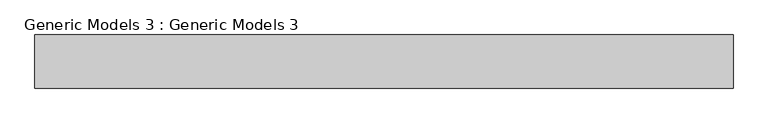
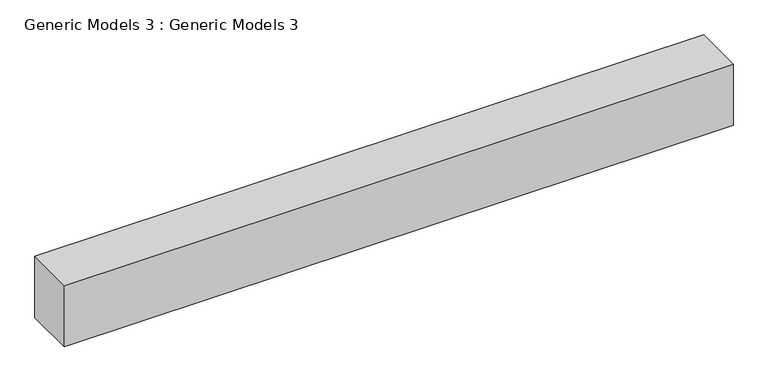
"""IFC4 building model written with IfcOpenShell, lengths in millimetres: proxy geometry, Generic Models 3 : Generic Models 3."""

from ifc_helpers import new_model, si_unit, frame, origin, place, context, project, spatial, polyline, outline, extrude, source, transform, mapped, element, save


def generic_models_3_generic_models_3_f2888e8d(model_context):
    return source(origin(), model_context, "Body", "SweptSolid", [
        extrude(outline(polyline([(3182.6580326, -8748.6246681), (3182.6580326, -9756.3414097), (-10060.7625896, -9756.3414097), (-10060.7625896, -8748.6246681), (3182.6580326, -8748.6246681)])), frame((0.0, 0.0, 6180.4335759), z_axis=(0.0, 0.0, 1.0), x_axis=(1.0, 0.0, 0.0)), (0.0, 0.0, 1.0), 1280.9305143),
    ])


if __name__ == "__main__":
    model = new_model("IFC4")
    model_context = context("Model", 3, world=origin())
    ifc_project = project(units=[si_unit("LENGTHUNIT", "METRE", prefix="MILLI")], contexts=[model_context])
    site = spatial("IfcSite", under=ifc_project)
    building = spatial("IfcBuilding", under=site)
    placement = place(None, origin())
    generic_models_3_generic_models_3_shape = generic_models_3_generic_models_3_f2888e8d(model_context)
    element("IfcBuildingElementProxy", 1, Name="Generic Models 3 : Generic Models 3", ObjectType="Generic Models 3 : Generic Models 3", at=placement, inside=building, context=model_context, shape_type="MappedRepresentation", body=[
        mapped(generic_models_3_generic_models_3_shape, transform((0.0, 0.0, 0.0), x_axis=(1.0, 0.0, 0.0), y_axis=(0.0, 1.0, 0.0), z_axis=(0.0, 0.0, 1.0))),
    ])
    save(model, "model.ifc")
